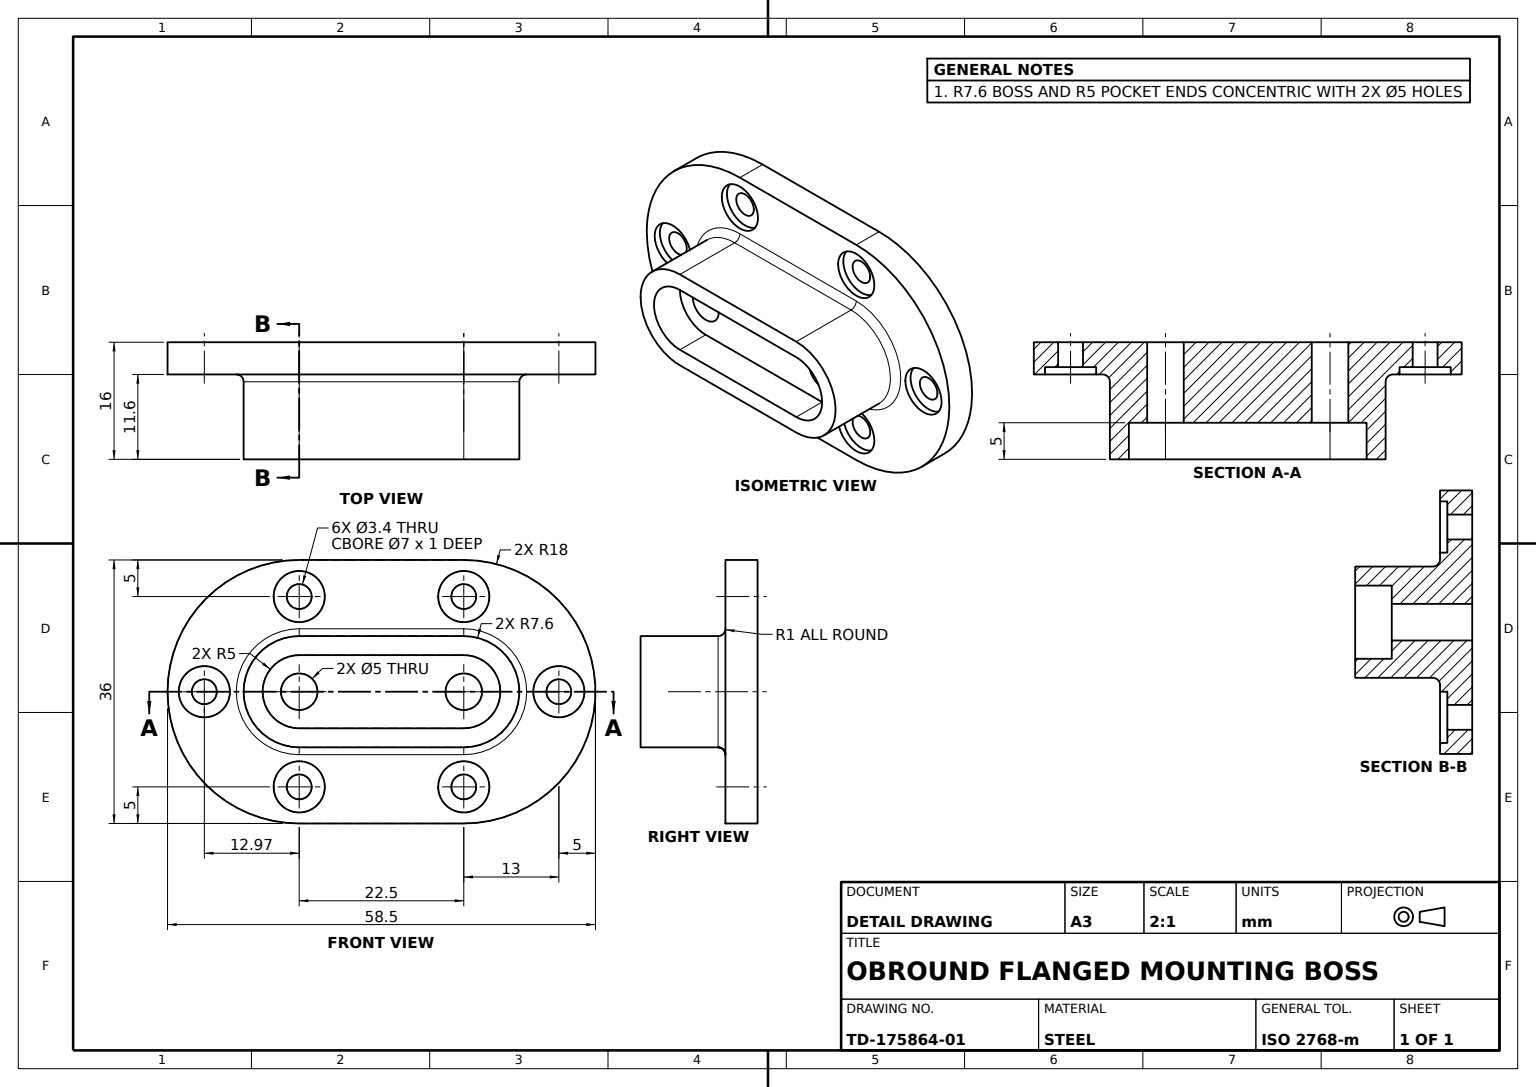
SolidWorks part; units mm, degrees
material "Plain Carbon Steel"
ref_plane "Front Plane" through (0, 0, 0) normal (0, 0, 1) x (1, 0, 0)
ref_plane "Top Plane" through (0, 0, 0) normal (0, 1, 0) x (1, 0, 0)
ref_plane "Right Plane" through (0, 0, 0) normal (1, 0, 0) x (0, 0, -1)
sketch "Flange Profile Sketch" plane through (0, 0, 0) normal (0, 0, 1) x (1, 0, 0)
  line L0 (-11.25, 0) -> (11.25, 0) construction
  line L1 (-11.25, 18) -> (11.25, 18)
  line L2 (-11.25, -18) -> (11.25, -18)
  arc A0 (-11.25, 18) -> (-11.25, -18) centre (-11.25, 0) ccw
  arc A1 (11.25, -18) -> (11.25, 18) centre (11.25, 0) ccw
  point P2 (0, 0)
  dimension "D2" = 18
  dimension "D1" = 22.5
extrude "Oval Base Flange" add sketch "Flange Profile Sketch" along normal blind 4.4
sketch "Housing Profile Sketch" plane through (0, 0, 4.4) normal (0, 0, 1) x (1, 0, 0)
  line L0 (-11.25, 0) -> (11.25, 0) construction
  line L1 (-11.25, 7.6) -> (11.25, 7.6)
  line L2 (-11.25, -7.6) -> (11.25, -7.6)
  arc A0 (-11.25, 7.6) -> (-11.25, -7.6) centre (-11.25, 0) ccw
  arc A1 (11.25, -7.6) -> (11.25, 7.6) centre (11.25, 0) ccw
  point P2 (0, 0)
  dimension "D2" = 7.6
  dimension "D1" = 22.5
extrude "Raised Obround Housing" add sketch "Housing Profile Sketch" along normal blind 11.6
sketch "Housing Slot Sketch" plane through (0, 0, 16) normal (0, 0, 1) x (1, 0, 0)
  line L0 (-11.25, 0) -> (11.25, 0) construction
  line L1 (-11.25, 5) -> (11.25, 5)
  line L2 (-11.25, -5) -> (11.25, -5)
  arc A0 (-11.25, 5) -> (-11.25, -5) centre (-11.25, 0) ccw
  arc A1 (11.25, -5) -> (11.25, 5) centre (11.25, 0) ccw
  point P2 (0, 0)
  dimension "D2" = 5
  dimension "D1" = 22.5
extrude "Housing Slot R5" cut sketch "Housing Slot Sketch" against normal blind 5
sketch "Mounting Holes Sketch" plane through (0, 0, 4.4) normal (0, 0, 1) x (1, 0, 0)
  line L0 (0, 0) -> (-29.25, 0) construction
  line L1 (0, 0) -> (29.25, 0) construction
  line L2 (-11.25, 0) -> (-11.25, 18) construction
  line L3 (-11.25, 0) -> (-11.25, -18) construction
  line L4 (11.25, 0) -> (11.25, 18) construction
  line L5 (11.25, 0) -> (11.25, -18) construction
  line L6 (-11.25, 0) -> (11.25, 0) construction
  line L7 (-11.25, 13) -> (11.25, 13) construction
  line L8 (-11.25, -13) -> (11.25, -13) construction
  arc A0 (-11.25, 18) -> (-11.25, -18) centre (-11.25, 0) ccw construction
  arc A1 (11.25, -18) -> (11.25, 18) centre (11.25, 0) ccw construction
  arc A2 (-11.25, 13) -> (-11.25, -13) centre (-11.25, 0) ccw construction
  arc A3 (11.25, -13) -> (11.25, 13) centre (11.25, 0) ccw construction
  circle A4 centre (-24.222, 0) radius 1.7
  circle A5 centre (-11.25, 13) radius 1.7
  circle A6 centre (11.25, 13) radius 1.7
  circle A7 centre (24.25, 0) radius 1.7
  circle A8 centre (11.25, -13) radius 1.7
  circle A9 centre (-11.25, -13) radius 1.7
  point P23 (0, 0)
  dimension "D1" = 13
  dimension "D2" = 3.4
  dimension "D3" = 3.4
  dimension "D4" = 3.4
  dimension "D5" = 3.4
  dimension "D6" = 3.4
  dimension "D7" = 3.4
  dimension "D8" = 12.972
extrude "Mounting Holes 6xØ3.4" cut sketch "Mounting Holes Sketch" against normal blind 5
sketch "Counterbore Sketch" plane through (0, 0, 4.4) normal (0, 0, 1) x (1, 0, 0)
  circle A0 centre (-24.222, 0) radius 3.5
  circle A1 centre (-11.25, 13) radius 3.5
  circle A2 centre (11.25, 13) radius 3.5
  circle A3 centre (24.25, 0) radius 3.5
  circle A4 centre (11.25, -13) radius 3.5
  circle A5 centre (-11.25, -13) radius 3.5
  dimension "D1" = 7
  dimension "D2" = 7
  dimension "D3" = 7
  dimension "D4" = 7
  dimension "D5" = 7
  dimension "D6" = 7
extrude "Counterbores 6xØ7" cut sketch "Counterbore Sketch" against normal blind 1
sketch "Slot Through Cut Sketch" plane through (0, 0, 11) normal (0, 0, 1) x (1, 0, 0)
  circle A0 centre (-11.25, 0) radius 2.5
  circle A1 centre (11.25, 0) radius 2.5
  dimension "D1" = 5
  dimension "D2" = 5
extrude "Slot Through Cut" cut sketch "Slot Through Cut Sketch" against normal through all
fillet "Housing Base Fillet R1" radius 1 4 edges at (-18.85, 0, 4.4) (0, 7.6, 4.4) (18.85, 0, 4.4) (0, -7.6, 4.4)
